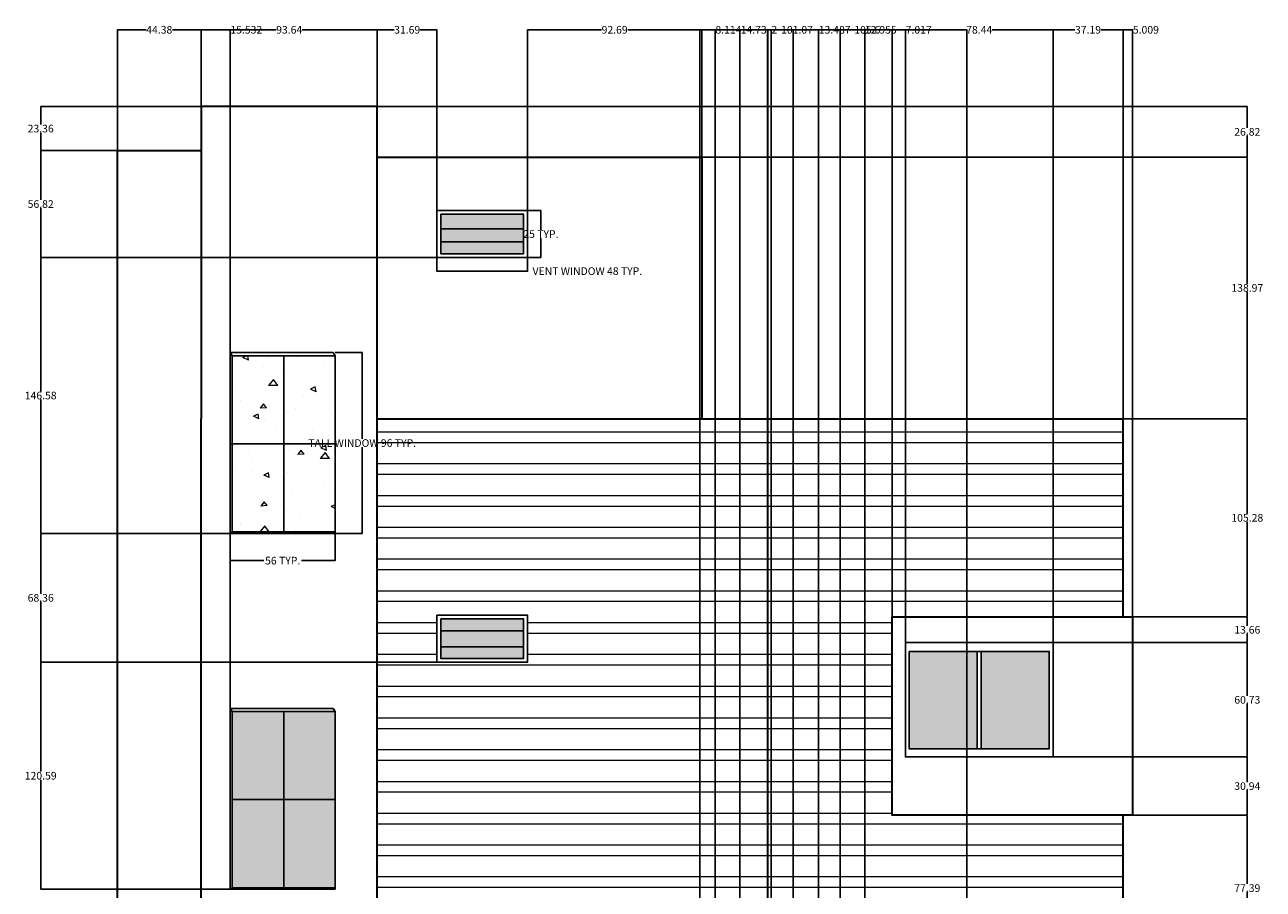
# Model space of a CAD drawing. Units: inches. Extents: x -35 to 623, y 74 to 964.
# Tile 3 of 3: x -35 to 623, y 505 to 964. Entities that reach past the tile are written whole.
import ezdxf

# ---------------------------------------------------------------- set-up
doc = ezdxf.new("R2010")
doc.units = ezdxf.units.IN
doc.header["$MEASUREMENT"] = 0
for name, color, linetype, lineweight in [('A-ANNO-DIMS', 2, 'Continuous', 18), ('A-ELEV', 7, 'Continuous', 35), ('A-ELEV-PATT', 8, 'Continuous', 13), ('A-GLAZ', 4, 'Continuous', 25)]:
    doc.layers.add(name, color=color, linetype=linetype, lineweight=lineweight)
doc.styles.get("Standard").update_dxf_attribs({"font": 'arial.ttf'})
doc.dimstyles.get("Standard").update_dxf_attribs({"dimtxt": 4.0625, "dimasz": 0.18, "dimexe": 0.18, "dimexo": 0.0625, "dimgap": 0.09, "dimtad": 0, "dimtih": 1, "dimtoh": 1, "dimdec": 4, "dimzin": 0, "dimdsep": 46, "dimlunit": 4, "dimtxsty": 'Standard', "dimcen": 0.09, "dimadec": 0, "dimazin": 0, "dimtfac": 1, "dimtdec": 4, "dimtofl": 0, "dimtmove": 0, "dimatfit": 3, "dimfxl": 1, "dimtolj": 1, "dimtzin": 0, "dimarcsym": 0})

# ---------------------------------------------------------------- blocks, each defined once
blk = doc.blocks.new('WIN-TALL-2X2')
for p, q in [((1.05, 94.39), (0, 96.09)), ((0, 96.09), (0, 0)), ((54.58, 96.06), (0, 96.06)), ((28.36, 94.39), (28.36, 0.82)), ((55.68, 94.39), (54.58, 96.06)), ((1.05, 0.82), (0, 0)), ((55.68, 0.82), (55.68, 0)), ((0, 0), (55.68, 0))]:
    blk.add_line(p, q)
blk.add_lwpolyline([(1.05, 94.39), (55.68, 94.39), (55.68, 0.82), (1.05, 0.82)], close=True)
blk = doc.blocks.new('VENT-FRAME')
for points in [[(0, 25.02), (48.03, 25.02), (48.03, 0), (0, 0)], [(2, 23.02), (46.03, 23.02), (46.03, 2), (2, 2)]]:
    blk.add_lwpolyline(points, close=True)
blk = doc.blocks.new('*D5')
at = {"layer": 'A-ANNO-DIMS', "color": 0, "lineweight": -2, "transparency": 16777216}
for p, q in [((129.92, 790.25), (144.45, 790.25)), ((144.27, 790.07), (144.27, 744.4)), ((144.27, 694.34), (144.27, 740.01)), ((129.92, 694.16), (144.45, 694.16))]:
    blk.add_line(p, q, dxfattribs=at)
at = {"layer": 'A-ANNO-DIMS', "color": 0, "transparency": 16777216}
for points in [[(144.24, 790.07), (144.3, 790.07), (144.27, 790.25)], [(144.24, 694.34), (144.3, 694.34), (144.27, 694.16)]]:
    blk.add_solid(points, dxfattribs=at)
at = {"layer": 'Defpoints', "color": 0, "transparency": 16777216}
for p in [(129.85, 790.25), (144.27, 790.25), (129.85, 694.16)]:
    blk.add_point(p, dxfattribs=at)
at = {"layer": 'A-ANNO-DIMS', "color": 0, "transparency": 16777216, "insert": (144.27, 742.2), "char_height": 4.0625, "attachment_point": 5}
blk.add_mtext('\\A1;TALL WINDOW 96 TYP.', dxfattribs=at)
blk = doc.blocks.new('*D6')
at = {"layer": 'A-ANNO-DIMS', "color": 0, "lineweight": -2, "transparency": 16777216}
for p, q in [((74.18, 694.1), (74.18, 679.56)), ((129.85, 694.1), (129.85, 679.56)), ((74.36, 679.74), (92.04, 679.74)), ((129.67, 679.74), (111.99, 679.74))]:
    blk.add_line(p, q, dxfattribs=at)
at = {"layer": 'A-ANNO-DIMS', "color": 0, "transparency": 16777216}
for points in [[(74.36, 679.77), (74.36, 679.71), (74.18, 679.74)], [(129.67, 679.77), (129.67, 679.71), (129.85, 679.74)]]:
    blk.add_solid(points, dxfattribs=at)
at = {"layer": 'Defpoints', "color": 0, "transparency": 16777216}
for p in [(74.18, 694.16), (129.85, 694.16), (129.85, 679.74)]:
    blk.add_point(p, dxfattribs=at)
at = {"layer": 'A-ANNO-DIMS', "color": 0, "transparency": 16777216, "insert": (102.02, 679.74), "char_height": 4.0625, "attachment_point": 5}
blk.add_mtext('\\A1;56 TYP.', dxfattribs=at)
blk = doc.blocks.new('*D7')
at = {"layer": 'A-ANNO-DIMS', "color": 0, "lineweight": -2, "transparency": 16777216}
for p, q in [((183.98, 840.67), (183.98, 833.35)), ((232.01, 840.67), (232.01, 833.35)), ((184.16, 833.53), (231.83, 833.53)), ((232.01, 833.53), (232.19, 833.53))]:
    blk.add_line(p, q, dxfattribs=at)
at = {"layer": 'A-ANNO-DIMS', "color": 0, "transparency": 16777216}
for points in [[(184.16, 833.56), (184.16, 833.5), (183.98, 833.53)], [(231.83, 833.56), (231.83, 833.5), (232.01, 833.53)]]:
    blk.add_solid(points, dxfattribs=at)
at = {"layer": 'Defpoints', "color": 0, "transparency": 16777216}
for p in [(183.98, 840.73), (232.01, 840.73), (232.01, 833.53)]:
    blk.add_point(p, dxfattribs=at)
at = {"layer": 'A-ANNO-DIMS', "color": 0, "transparency": 16777216, "insert": (263.87, 833.53), "char_height": 4.0625, "attachment_point": 5}
blk.add_mtext('\\A1;VENT WINDOW 48 TYP.', dxfattribs=at)
blk = doc.blocks.new('*D8')
at = {"layer": 'A-ANNO-DIMS', "color": 0, "lineweight": -2, "transparency": 16777216}
for p, q in [((232.07, 865.75), (239.39, 865.75)), ((239.21, 865.57), (239.21, 855.41)), ((239.21, 840.91), (239.21, 851.08)), ((232.07, 840.73), (239.39, 840.73))]:
    blk.add_line(p, q, dxfattribs=at)
at = {"layer": 'A-ANNO-DIMS', "color": 0, "transparency": 16777216}
for points in [[(239.18, 865.57), (239.24, 865.57), (239.21, 865.75)], [(239.18, 840.91), (239.24, 840.91), (239.21, 840.73)]]:
    blk.add_solid(points, dxfattribs=at)
at = {"layer": 'Defpoints', "color": 0, "transparency": 16777216}
for p in [(232.01, 865.75), (239.21, 865.75), (232.01, 840.73)]:
    blk.add_point(p, dxfattribs=at)
at = {"layer": 'A-ANNO-DIMS', "color": 0, "transparency": 16777216, "insert": (239.21, 853.24), "char_height": 4.0625, "attachment_point": 5}
blk.add_mtext('\\A1;25 TYP.', dxfattribs=at)
blk = doc.blocks.new('*D14')
at = {"layer": 'A-ANNO-DIMS', "color": 0, "lineweight": -2, "transparency": 16777216}
for p, q in [((14.26, 897.62), (14.26, 961.9)), ((14.44, 961.72), (29.42, 961.72)), ((58.47, 961.72), (43.48, 961.72)), ((58.65, 920.98), (58.65, 961.9))]:
    blk.add_line(p, q, dxfattribs=at)
at = {"layer": 'A-ANNO-DIMS', "color": 0, "transparency": 16777216}
for points in [[(14.44, 961.75), (14.44, 961.69), (14.26, 961.72)], [(58.47, 961.75), (58.47, 961.69), (58.65, 961.72)]]:
    blk.add_solid(points, dxfattribs=at)
at = {"layer": 'Defpoints', "color": 0, "transparency": 16777216}
for p in [(58.65, 961.72), (58.65, 920.92), (14.26, 897.56)]:
    blk.add_point(p, dxfattribs=at)
at = {"layer": 'A-ANNO-DIMS', "color": 0, "transparency": 16777216, "insert": (36.45, 961.72), "char_height": 4.062, "attachment_point": 5}
blk.add_mtext('\\A1;44.38', dxfattribs=at)
blk = doc.blocks.new('*D15')
at = {"layer": 'A-ANNO-DIMS', "color": 0, "lineweight": -2, "transparency": 16777216}
for p, q in [((58.65, 920.98), (58.65, 961.9)), ((58.83, 961.72), (98.53, 961.72)), ((152.11, 961.72), (112.4, 961.72)), ((152.29, 920.98), (152.29, 961.9))]:
    blk.add_line(p, q, dxfattribs=at)
at = {"layer": 'A-ANNO-DIMS', "color": 0, "transparency": 16777216}
for points in [[(58.83, 961.75), (58.83, 961.69), (58.65, 961.72)], [(152.11, 961.75), (152.11, 961.69), (152.29, 961.72)]]:
    blk.add_solid(points, dxfattribs=at)
at = {"layer": 'Defpoints', "color": 0, "transparency": 16777216}
for p in [(152.29, 961.72), (58.65, 920.92), (152.29, 920.92)]:
    blk.add_point(p, dxfattribs=at)
at = {"layer": 'A-ANNO-DIMS', "color": 0, "transparency": 16777216, "insert": (105.47, 961.72), "char_height": 4.062, "attachment_point": 5}
blk.add_mtext('\\A1;93.64', dxfattribs=at)
blk = doc.blocks.new('*D16')
at = {"layer": 'A-ANNO-DIMS', "color": 0, "lineweight": -2, "transparency": 16777216}
for p, q in [((152.29, 894.16), (152.29, 961.9)), ((152.47, 961.72), (161.19, 961.72)), ((183.8, 961.72), (175.08, 961.72)), ((183.98, 865.81), (183.98, 961.9))]:
    blk.add_line(p, q, dxfattribs=at)
at = {"layer": 'A-ANNO-DIMS', "color": 0, "transparency": 16777216}
for points in [[(152.47, 961.75), (152.47, 961.69), (152.29, 961.72)], [(183.8, 961.75), (183.8, 961.69), (183.98, 961.72)]]:
    blk.add_solid(points, dxfattribs=at)
at = {"layer": 'Defpoints', "color": 0, "transparency": 16777216}
for p in [(183.98, 961.72), (152.29, 894.1), (183.98, 865.75)]:
    blk.add_point(p, dxfattribs=at)
at = {"layer": 'A-ANNO-DIMS', "color": 0, "transparency": 16777216, "insert": (168.14, 961.72), "char_height": 4.062, "attachment_point": 5}
blk.add_mtext('\\A1;31.69', dxfattribs=at)
blk = doc.blocks.new('*D17')
at = {"layer": 'A-ANNO-DIMS', "color": 0, "lineweight": -2, "transparency": 16777216}
for p, q in [((232.01, 865.81), (232.01, 961.9)), ((232.19, 961.72), (271.4, 961.72)), ((324.52, 961.72), (285.3, 961.72)), ((324.7, 894.16), (324.7, 961.9))]:
    blk.add_line(p, q, dxfattribs=at)
at = {"layer": 'A-ANNO-DIMS', "color": 0, "transparency": 16777216}
for points in [[(232.19, 961.75), (232.19, 961.69), (232.01, 961.72)], [(324.52, 961.75), (324.52, 961.69), (324.7, 961.72)]]:
    blk.add_solid(points, dxfattribs=at)
at = {"layer": 'Defpoints', "color": 0, "transparency": 16777216}
for p in [(324.7, 961.72), (324.7, 894.1), (232.01, 865.75)]:
    blk.add_point(p, dxfattribs=at)
at = {"layer": 'A-ANNO-DIMS', "color": 0, "transparency": 16777216, "insert": (278.35, 961.72), "char_height": 4.062, "attachment_point": 5}
blk.add_mtext('\\A1;92.69', dxfattribs=at)
blk = doc.blocks.new('*D18')
at = {"layer": 'A-ANNO-DIMS', "color": 0, "lineweight": -2, "transparency": 16777216}
for p, q in [((324.7, 755.19), (324.7, 961.9)), ((324.88, 961.72), (366.9, 961.72)), ((425.59, 961.72), (383.56, 961.72)), ((425.77, 649.91), (425.77, 961.9))]:
    blk.add_line(p, q, dxfattribs=at)
at = {"layer": 'A-ANNO-DIMS', "color": 0, "transparency": 16777216}
for points in [[(324.88, 961.75), (324.88, 961.69), (324.7, 961.72)], [(425.59, 961.75), (425.59, 961.69), (425.77, 961.72)]]:
    blk.add_solid(points, dxfattribs=at)
at = {"layer": 'Defpoints', "color": 0, "transparency": 16777216}
for p in [(425.77, 961.72), (324.7, 755.13), (425.77, 649.84)]:
    blk.add_point(p, dxfattribs=at)
at = {"layer": 'A-ANNO-DIMS', "color": 0, "transparency": 16777216, "insert": (375.23, 961.72), "char_height": 4.062, "attachment_point": 5}
blk.add_mtext('\\A1;101.07', dxfattribs=at)
blk = doc.blocks.new('*D19')
at = {"layer": 'A-ANNO-DIMS', "color": 0, "lineweight": -2, "transparency": 16777216}
for p, q in [((425.77, 649.91), (425.77, 961.9)), ((425.95, 961.72), (432.61, 961.72)), ((432.79, 636.25), (432.79, 961.9)), ((432.79, 961.72), (432.97, 961.72))]:
    blk.add_line(p, q, dxfattribs=at)
at = {"layer": 'A-ANNO-DIMS', "color": 0, "transparency": 16777216}
for points in [[(425.95, 961.75), (425.95, 961.69), (425.77, 961.72)], [(432.61, 961.75), (432.61, 961.69), (432.79, 961.72)]]:
    blk.add_solid(points, dxfattribs=at)
at = {"layer": 'Defpoints', "color": 0, "transparency": 16777216}
for p in [(432.79, 961.72), (425.77, 649.84), (432.79, 636.18)]:
    blk.add_point(p, dxfattribs=at)
at = {"layer": 'A-ANNO-DIMS', "color": 0, "transparency": 16777216, "insert": (439.89, 961.72), "char_height": 4.062, "attachment_point": 5}
blk.add_mtext('\\A1;7.017', dxfattribs=at)
blk = doc.blocks.new('*D20')
at = {"layer": 'A-ANNO-DIMS', "color": 0, "lineweight": -2, "transparency": 16777216}
for p, q in [((432.79, 636.25), (432.79, 961.9)), ((432.97, 961.72), (465.09, 961.72)), ((511.05, 961.72), (478.93, 961.72)), ((511.23, 636.25), (511.23, 961.9))]:
    blk.add_line(p, q, dxfattribs=at)
at = {"layer": 'A-ANNO-DIMS', "color": 0, "transparency": 16777216}
for points in [[(432.97, 961.75), (432.97, 961.69), (432.79, 961.72)], [(511.05, 961.75), (511.05, 961.69), (511.23, 961.72)]]:
    blk.add_solid(points, dxfattribs=at)
at = {"layer": 'Defpoints', "color": 0, "transparency": 16777216}
for p in [(511.23, 961.72), (432.79, 636.18), (511.23, 636.18)]:
    blk.add_point(p, dxfattribs=at)
at = {"layer": 'A-ANNO-DIMS', "color": 0, "transparency": 16777216, "insert": (472.01, 961.72), "char_height": 4.062, "attachment_point": 5}
blk.add_mtext('\\A1;78.44', dxfattribs=at)
blk = doc.blocks.new('*D21')
at = {"layer": 'A-ANNO-DIMS', "color": 0, "lineweight": -2, "transparency": 16777216}
for p, q in [((511.23, 636.25), (511.23, 961.9)), ((511.41, 961.72), (522.87, 961.72)), ((548.24, 961.72), (536.77, 961.72)), ((548.42, 755.19), (548.42, 961.9))]:
    blk.add_line(p, q, dxfattribs=at)
at = {"layer": 'A-ANNO-DIMS', "color": 0, "transparency": 16777216}
for points in [[(511.41, 961.75), (511.41, 961.69), (511.23, 961.72)], [(548.24, 961.75), (548.24, 961.69), (548.42, 961.72)]]:
    blk.add_solid(points, dxfattribs=at)
at = {"layer": 'Defpoints', "color": 0, "transparency": 16777216}
for p in [(548.42, 961.72), (548.42, 755.13), (511.23, 636.18)]:
    blk.add_point(p, dxfattribs=at)
at = {"layer": 'A-ANNO-DIMS', "color": 0, "transparency": 16777216, "insert": (529.82, 961.72), "char_height": 4.062, "attachment_point": 5}
blk.add_mtext('\\A1;37.19', dxfattribs=at)
blk = doc.blocks.new('*D22')
at = {"layer": 'A-ANNO-DIMS', "color": 0, "lineweight": -2, "transparency": 16777216}
for p, q in [((548.42, 755.19), (548.42, 961.9)), ((548.6, 961.72), (553.25, 961.72)), ((553.43, 649.91), (553.43, 961.9)), ((553.43, 961.72), (553.61, 961.72))]:
    blk.add_line(p, q, dxfattribs=at)
at = {"layer": 'A-ANNO-DIMS', "color": 0, "transparency": 16777216}
for points in [[(548.6, 961.75), (548.6, 961.69), (548.42, 961.72)], [(553.25, 961.75), (553.25, 961.69), (553.43, 961.72)]]:
    blk.add_solid(points, dxfattribs=at)
at = {"layer": 'Defpoints', "color": 0, "transparency": 16777216}
for p in [(553.43, 961.72), (548.42, 755.13), (553.43, 649.84)]:
    blk.add_point(p, dxfattribs=at)
at = {"layer": 'A-ANNO-DIMS', "color": 0, "transparency": 16777216, "insert": (560.56, 961.72), "char_height": 4.062, "attachment_point": 5}
blk.add_mtext('\\A1;5.009', dxfattribs=at)
blk = doc.blocks.new('*D26')
at = {"layer": 'A-ANNO-DIMS', "color": 0, "lineweight": -2, "transparency": 16777216}
for p, q in [((553.49, 544.52), (614.62, 544.52)), ((614.44, 544.34), (614.44, 507.99)), ((614.44, 467.31), (614.44, 503.66)), ((548.48, 467.13), (614.62, 467.13))]:
    blk.add_line(p, q, dxfattribs=at)
at = {"layer": 'A-ANNO-DIMS', "color": 0, "transparency": 16777216}
for points in [[(614.41, 544.34), (614.47, 544.34), (614.44, 544.52)], [(614.41, 467.31), (614.47, 467.31), (614.44, 467.13)]]:
    blk.add_solid(points, dxfattribs=at)
at = {"layer": 'Defpoints', "color": 0, "transparency": 16777216}
for p in [(553.43, 544.52), (614.44, 544.52), (548.42, 467.13)]:
    blk.add_point(p, dxfattribs=at)
at = {"layer": 'A-ANNO-DIMS', "color": 0, "transparency": 16777216, "insert": (614.44, 505.82), "char_height": 4.062, "attachment_point": 5}
blk.add_mtext('\\A1;77.39', dxfattribs=at)
blk = doc.blocks.new('*D27')
at = {"layer": 'A-ANNO-DIMS', "color": 0, "lineweight": -2, "transparency": 16777216}
for p, q in [((511.29, 575.46), (614.62, 575.46)), ((614.44, 575.28), (614.44, 562.15)), ((614.44, 544.7), (614.44, 557.82)), ((553.49, 544.52), (614.62, 544.52))]:
    blk.add_line(p, q, dxfattribs=at)
at = {"layer": 'A-ANNO-DIMS', "color": 0, "transparency": 16777216}
for points in [[(614.41, 575.28), (614.47, 575.28), (614.44, 575.46)], [(614.41, 544.7), (614.47, 544.7), (614.44, 544.52)]]:
    blk.add_solid(points, dxfattribs=at)
at = {"layer": 'Defpoints', "color": 0, "transparency": 16777216}
for p in [(511.23, 575.46), (614.44, 575.46), (553.43, 544.52)]:
    blk.add_point(p, dxfattribs=at)
at = {"layer": 'A-ANNO-DIMS', "color": 0, "transparency": 16777216, "insert": (614.44, 559.99), "char_height": 4.062, "attachment_point": 5}
blk.add_mtext('\\A1;30.94', dxfattribs=at)
blk = doc.blocks.new('*D28')
at = {"layer": 'A-ANNO-DIMS', "color": 0, "lineweight": -2, "transparency": 16777216}
for p, q in [((511.29, 636.18), (614.62, 636.18)), ((614.44, 636), (614.44, 607.98)), ((614.44, 575.64), (614.44, 603.65)), ((511.29, 575.46), (614.62, 575.46))]:
    blk.add_line(p, q, dxfattribs=at)
at = {"layer": 'A-ANNO-DIMS', "color": 0, "transparency": 16777216}
for points in [[(614.41, 636), (614.47, 636), (614.44, 636.18)], [(614.41, 575.64), (614.47, 575.64), (614.44, 575.46)]]:
    blk.add_solid(points, dxfattribs=at)
at = {"layer": 'Defpoints', "color": 0, "transparency": 16777216}
for p in [(511.23, 636.18), (614.44, 636.18), (511.23, 575.46)]:
    blk.add_point(p, dxfattribs=at)
at = {"layer": 'A-ANNO-DIMS', "color": 0, "transparency": 16777216, "insert": (614.44, 605.82), "char_height": 4.062, "attachment_point": 5}
blk.add_mtext('\\A1;60.73', dxfattribs=at)
blk = doc.blocks.new('*D29')
at = {"layer": 'A-ANNO-DIMS', "color": 0, "lineweight": -2, "transparency": 16777216}
for p, q in [((553.49, 649.84), (614.62, 649.84)), ((614.44, 649.66), (614.44, 645.18)), ((614.44, 636.36), (614.44, 640.85)), ((511.29, 636.18), (614.62, 636.18))]:
    blk.add_line(p, q, dxfattribs=at)
at = {"layer": 'A-ANNO-DIMS', "color": 0, "transparency": 16777216}
for points in [[(614.41, 649.66), (614.47, 649.66), (614.44, 649.84)], [(614.41, 636.36), (614.47, 636.36), (614.44, 636.18)]]:
    blk.add_solid(points, dxfattribs=at)
at = {"layer": 'Defpoints', "color": 0, "transparency": 16777216}
for p in [(553.43, 649.84), (614.44, 649.84), (511.23, 636.18)]:
    blk.add_point(p, dxfattribs=at)
at = {"layer": 'A-ANNO-DIMS', "color": 0, "transparency": 16777216, "insert": (614.44, 643.01), "char_height": 4.062, "attachment_point": 5}
blk.add_mtext('\\A1;13.66', dxfattribs=at)
blk = doc.blocks.new('*D30')
at = {"layer": 'A-ANNO-DIMS', "color": 0, "lineweight": -2, "transparency": 16777216}
for p, q in [((548.48, 755.13), (614.62, 755.13)), ((614.44, 754.95), (614.44, 704.65)), ((614.44, 650.02), (614.44, 700.32)), ((553.49, 649.84), (614.62, 649.84))]:
    blk.add_line(p, q, dxfattribs=at)
at = {"layer": 'A-ANNO-DIMS', "color": 0, "transparency": 16777216}
for points in [[(614.41, 754.95), (614.47, 754.95), (614.44, 755.13)], [(614.41, 650.02), (614.47, 650.02), (614.44, 649.84)]]:
    blk.add_solid(points, dxfattribs=at)
at = {"layer": 'Defpoints', "color": 0, "transparency": 16777216}
for p in [(548.42, 755.13), (614.44, 755.13), (553.43, 649.84)]:
    blk.add_point(p, dxfattribs=at)
at = {"layer": 'A-ANNO-DIMS', "color": 0, "transparency": 16777216, "insert": (614.44, 702.49), "char_height": 4.062, "attachment_point": 5}
blk.add_mtext('\\A1;105.28', dxfattribs=at)
blk = doc.blocks.new('*D31')
at = {"layer": 'A-ANNO-DIMS', "color": 0, "lineweight": -2, "transparency": 16777216}
for p, q in [((324.76, 894.1), (614.62, 894.1)), ((614.44, 893.92), (614.44, 826.78)), ((614.44, 755.31), (614.44, 822.45)), ((548.48, 755.13), (614.62, 755.13))]:
    blk.add_line(p, q, dxfattribs=at)
at = {"layer": 'A-ANNO-DIMS', "color": 0, "transparency": 16777216}
for points in [[(614.41, 893.92), (614.47, 893.92), (614.44, 894.1)], [(614.41, 755.31), (614.47, 755.31), (614.44, 755.13)]]:
    blk.add_solid(points, dxfattribs=at)
at = {"layer": 'Defpoints', "color": 0, "transparency": 16777216}
for p in [(324.7, 894.1), (614.44, 894.1), (548.42, 755.13)]:
    blk.add_point(p, dxfattribs=at)
at = {"layer": 'A-ANNO-DIMS', "color": 0, "transparency": 16777216, "insert": (614.44, 824.61), "char_height": 4.062, "attachment_point": 5}
blk.add_mtext('\\A1;138.97', dxfattribs=at)
blk = doc.blocks.new('*D32')
at = {"layer": 'A-ANNO-DIMS', "color": 0, "lineweight": -2, "transparency": 16777216}
for p, q in [((152.35, 920.92), (614.62, 920.92)), ((614.44, 920.74), (614.44, 909.67)), ((614.44, 894.28), (614.44, 905.34)), ((324.76, 894.1), (614.62, 894.1))]:
    blk.add_line(p, q, dxfattribs=at)
at = {"layer": 'A-ANNO-DIMS', "color": 0, "transparency": 16777216}
for points in [[(614.41, 920.74), (614.47, 920.74), (614.44, 920.92)], [(614.41, 894.28), (614.47, 894.28), (614.44, 894.1)]]:
    blk.add_solid(points, dxfattribs=at)
at = {"layer": 'Defpoints', "color": 0, "transparency": 16777216}
for p in [(152.29, 920.92), (614.44, 920.92), (324.7, 894.1)]:
    blk.add_point(p, dxfattribs=at)
at = {"layer": 'A-ANNO-DIMS', "color": 0, "transparency": 16777216, "insert": (614.44, 907.51), "char_height": 4.062, "attachment_point": 5}
blk.add_mtext('\\A1;26.82', dxfattribs=at)
blk = doc.blocks.new('*D36')
at = {"layer": 'A-ANNO-DIMS', "color": 0, "lineweight": -2, "transparency": 16777216}
for p, q in [((183.92, 625.8), (-26.72, 625.8)), ((-26.54, 625.62), (-26.54, 567.67)), ((-26.54, 505.39), (-26.54, 563.34)), ((74.11, 505.21), (-26.72, 505.21))]:
    blk.add_line(p, q, dxfattribs=at)
at = {"layer": 'A-ANNO-DIMS', "color": 0, "transparency": 16777216}
for points in [[(-26.57, 625.62), (-26.51, 625.62), (-26.54, 625.8)], [(-26.57, 505.39), (-26.51, 505.39), (-26.54, 505.21)]]:
    blk.add_solid(points, dxfattribs=at)
at = {"layer": 'Defpoints', "color": 0, "transparency": 16777216}
for p in [(-26.54, 625.8), (183.98, 625.8), (74.18, 505.21)]:
    blk.add_point(p, dxfattribs=at)
at = {"layer": 'A-ANNO-DIMS', "color": 0, "transparency": 16777216, "insert": (-26.54, 565.5), "char_height": 4.062, "attachment_point": 5}
blk.add_mtext('\\A1;120.59', dxfattribs=at)
blk = doc.blocks.new('*D37')
at = {"layer": 'A-ANNO-DIMS', "color": 0, "lineweight": -2, "transparency": 16777216}
for p, q in [((74.11, 694.16), (-26.72, 694.16)), ((-26.54, 693.98), (-26.54, 662.14)), ((-26.54, 625.98), (-26.54, 657.81)), ((183.92, 625.8), (-26.72, 625.8))]:
    blk.add_line(p, q, dxfattribs=at)
at = {"layer": 'A-ANNO-DIMS', "color": 0, "transparency": 16777216}
for points in [[(-26.57, 693.98), (-26.51, 693.98), (-26.54, 694.16)], [(-26.57, 625.98), (-26.51, 625.98), (-26.54, 625.8)]]:
    blk.add_solid(points, dxfattribs=at)
at = {"layer": 'Defpoints', "color": 0, "transparency": 16777216}
for p in [(-26.54, 694.16), (74.18, 694.16), (183.98, 625.8)]:
    blk.add_point(p, dxfattribs=at)
at = {"layer": 'A-ANNO-DIMS', "color": 0, "transparency": 16777216, "insert": (-26.54, 659.98), "char_height": 4.062, "attachment_point": 5}
blk.add_mtext('\\A1;68.36', dxfattribs=at)
blk = doc.blocks.new('*D38')
at = {"layer": 'A-ANNO-DIMS', "color": 0, "lineweight": -2, "transparency": 16777216}
for p, q in [((183.92, 840.73), (-26.72, 840.73)), ((-26.54, 840.55), (-26.54, 769.61)), ((-26.54, 694.34), (-26.54, 765.28)), ((74.11, 694.16), (-26.72, 694.16))]:
    blk.add_line(p, q, dxfattribs=at)
at = {"layer": 'A-ANNO-DIMS', "color": 0, "transparency": 16777216}
for points in [[(-26.57, 840.55), (-26.51, 840.55), (-26.54, 840.73)], [(-26.57, 694.34), (-26.51, 694.34), (-26.54, 694.16)]]:
    blk.add_solid(points, dxfattribs=at)
at = {"layer": 'Defpoints', "color": 0, "transparency": 16777216}
for p in [(-26.54, 840.73), (183.98, 840.73), (74.18, 694.16)]:
    blk.add_point(p, dxfattribs=at)
at = {"layer": 'A-ANNO-DIMS', "color": 0, "transparency": 16777216, "insert": (-26.54, 767.45), "char_height": 4.062, "attachment_point": 5}
blk.add_mtext('\\A1;146.58', dxfattribs=at)
blk = doc.blocks.new('*D39')
at = {"layer": 'A-ANNO-DIMS', "color": 0, "lineweight": -2, "transparency": 16777216}
for p, q in [((14.2, 897.56), (-26.72, 897.56)), ((-26.54, 897.38), (-26.54, 871.31)), ((-26.54, 840.91), (-26.54, 866.98)), ((183.92, 840.73), (-26.72, 840.73))]:
    blk.add_line(p, q, dxfattribs=at)
at = {"layer": 'A-ANNO-DIMS', "color": 0, "transparency": 16777216}
for points in [[(-26.57, 897.38), (-26.51, 897.38), (-26.54, 897.56)], [(-26.57, 840.91), (-26.51, 840.91), (-26.54, 840.73)]]:
    blk.add_solid(points, dxfattribs=at)
at = {"layer": 'Defpoints', "color": 0, "transparency": 16777216}
for p in [(-26.54, 897.56), (14.26, 897.56), (183.98, 840.73)]:
    blk.add_point(p, dxfattribs=at)
at = {"layer": 'A-ANNO-DIMS', "color": 0, "transparency": 16777216, "insert": (-26.54, 869.15), "char_height": 4.062, "attachment_point": 5}
blk.add_mtext('\\A1;56.82', dxfattribs=at)
blk = doc.blocks.new('*D40')
at = {"layer": 'A-ANNO-DIMS', "color": 0, "lineweight": -2, "transparency": 16777216}
for p, q in [((58.58, 920.92), (-26.72, 920.92)), ((-26.54, 920.74), (-26.54, 911.4)), ((-26.54, 897.74), (-26.54, 907.07)), ((14.2, 897.56), (-26.72, 897.56))]:
    blk.add_line(p, q, dxfattribs=at)
at = {"layer": 'A-ANNO-DIMS', "color": 0, "transparency": 16777216}
for points in [[(-26.57, 920.74), (-26.51, 920.74), (-26.54, 920.92)], [(-26.57, 897.74), (-26.51, 897.74), (-26.54, 897.56)]]:
    blk.add_solid(points, dxfattribs=at)
at = {"layer": 'Defpoints', "color": 0, "transparency": 16777216}
for p in [(-26.54, 920.92), (58.65, 920.92), (14.26, 897.56)]:
    blk.add_point(p, dxfattribs=at)
at = {"layer": 'A-ANNO-DIMS', "color": 0, "transparency": 16777216, "insert": (-26.54, 909.24), "char_height": 4.062, "attachment_point": 5}
blk.add_mtext('\\A1;23.36', dxfattribs=at)
blk = doc.blocks.new('*D41')
at = {"layer": 'A-ANNO-DIMS', "color": 0, "lineweight": -2, "transparency": 16777216}
for p, q in [((58.65, 611.19), (58.65, 961.9)), ((58.83, 961.72), (74, 961.72)), ((74.18, 601.33), (74.18, 961.9)), ((74.18, 961.72), (74.36, 961.72))]:
    blk.add_line(p, q, dxfattribs=at)
at = {"layer": 'A-ANNO-DIMS', "color": 0, "transparency": 16777216}
for points in [[(58.83, 961.75), (58.83, 961.69), (58.65, 961.72)], [(74, 961.75), (74, 961.69), (74.18, 961.72)]]:
    blk.add_solid(points, dxfattribs=at)
at = {"layer": 'Defpoints', "color": 0, "transparency": 16777216}
for p in [(74.18, 961.72), (58.65, 611.13), (74.18, 601.27)]:
    blk.add_point(p, dxfattribs=at)
at = {"layer": 'A-ANNO-DIMS', "color": 0, "transparency": 16777216, "insert": (82.67, 961.72), "char_height": 4.062, "attachment_point": 5}
blk.add_mtext('\\A1;15.532', dxfattribs=at)
blk = doc.blocks.new('*D58')
at = {"layer": 'A-ANNO-DIMS', "color": 0, "lineweight": -2, "transparency": 16777216}
for p, q in [((323.56, 323.19), (323.56, 961.9)), ((323.74, 961.72), (331.5, 961.72)), ((331.68, 323.19), (331.68, 961.9)), ((331.68, 961.72), (331.86, 961.72))]:
    blk.add_line(p, q, dxfattribs=at)
at = {"layer": 'A-ANNO-DIMS', "color": 0, "transparency": 16777216}
for points in [[(323.74, 961.75), (323.74, 961.69), (323.56, 961.72)], [(331.5, 961.75), (331.5, 961.69), (331.68, 961.72)]]:
    blk.add_solid(points, dxfattribs=at)
at = {"layer": 'Defpoints', "color": 0, "transparency": 16777216}
for p in [(331.68, 961.72), (323.56, 323.13), (331.68, 323.13)]:
    blk.add_point(p, dxfattribs=at)
at = {"layer": 'A-ANNO-DIMS', "color": 0, "transparency": 16777216, "insert": (338.8, 961.72), "char_height": 4.062, "attachment_point": 5}
blk.add_mtext('\\A1;8.114', dxfattribs=at)
blk = doc.blocks.new('*D59')
at = {"layer": 'A-ANNO-DIMS', "color": 0, "lineweight": -2, "transparency": 16777216}
for p, q in [((344.83, 323.19), (344.83, 961.9)), ((345.01, 961.72), (345.44, 961.72)), ((359.38, 961.72), (358.95, 961.72)), ((359.56, 323.19), (359.56, 961.9))]:
    blk.add_line(p, q, dxfattribs=at)
at = {"layer": 'A-ANNO-DIMS', "color": 0, "transparency": 16777216}
for points in [[(345.01, 961.75), (345.01, 961.69), (344.83, 961.72)], [(359.38, 961.75), (359.38, 961.69), (359.56, 961.72)]]:
    blk.add_solid(points, dxfattribs=at)
at = {"layer": 'Defpoints', "color": 0, "transparency": 16777216}
for p in [(359.56, 961.72), (344.83, 323.13), (359.56, 323.13)]:
    blk.add_point(p, dxfattribs=at)
at = {"layer": 'A-ANNO-DIMS', "color": 0, "transparency": 16777216, "insert": (352.19, 961.72), "char_height": 4.062, "attachment_point": 5}
blk.add_mtext('\\A1;14.73', dxfattribs=at)
blk = doc.blocks.new('*D60')
at = {"layer": 'A-ANNO-DIMS', "color": 0, "lineweight": -2, "transparency": 16777216}
for p, q in [((359.56, 323.19), (359.56, 961.9)), ((359.74, 961.72), (361.38, 961.72)), ((361.56, 323.19), (361.56, 961.9)), ((361.56, 961.72), (361.74, 961.72))]:
    blk.add_line(p, q, dxfattribs=at)
at = {"layer": 'A-ANNO-DIMS', "color": 0, "transparency": 16777216}
for points in [[(359.74, 961.75), (359.74, 961.69), (359.56, 961.72)], [(361.38, 961.75), (361.38, 961.69), (361.56, 961.72)]]:
    blk.add_solid(points, dxfattribs=at)
at = {"layer": 'Defpoints', "color": 0, "transparency": 16777216}
for p in [(361.56, 961.72), (359.56, 323.13), (361.56, 323.13)]:
    blk.add_point(p, dxfattribs=at)
at = {"layer": 'A-ANNO-DIMS', "color": 0, "transparency": 16777216, "insert": (363.17, 961.72), "char_height": 4.062, "attachment_point": 5}
blk.add_mtext('\\A1;2', dxfattribs=at)
blk = doc.blocks.new('*D61')
at = {"layer": 'A-ANNO-DIMS', "color": 0, "lineweight": -2, "transparency": 16777216}
for p, q in [((373.22, 323.19), (373.22, 961.9)), ((373.4, 961.72), (386.53, 961.72)), ((386.71, 323.19), (386.71, 961.9)), ((386.71, 961.72), (386.89, 961.72))]:
    blk.add_line(p, q, dxfattribs=at)
at = {"layer": 'A-ANNO-DIMS', "color": 0, "transparency": 16777216}
for points in [[(373.4, 961.75), (373.4, 961.69), (373.22, 961.72)], [(386.53, 961.75), (386.53, 961.69), (386.71, 961.72)]]:
    blk.add_solid(points, dxfattribs=at)
at = {"layer": 'Defpoints', "color": 0, "transparency": 16777216}
for p in [(386.71, 961.72), (373.22, 323.13), (386.71, 323.13)]:
    blk.add_point(p, dxfattribs=at)
at = {"layer": 'A-ANNO-DIMS', "color": 0, "transparency": 16777216, "insert": (395.22, 961.72), "char_height": 4.062, "attachment_point": 5}
blk.add_mtext('\\A1;13.487', dxfattribs=at)
blk = doc.blocks.new('*D62')
at = {"layer": 'A-ANNO-DIMS', "color": 0, "lineweight": -2, "transparency": 16777216}
for p, q in [((398.24, 323.19), (398.24, 961.9)), ((398.42, 961.72), (411.02, 961.72)), ((411.2, 323.19), (411.2, 961.9)), ((411.2, 961.72), (411.38, 961.72))]:
    blk.add_line(p, q, dxfattribs=at)
at = {"layer": 'A-ANNO-DIMS', "color": 0, "transparency": 16777216}
for points in [[(398.42, 961.75), (398.42, 961.69), (398.24, 961.72)], [(411.02, 961.75), (411.02, 961.69), (411.2, 961.72)]]:
    blk.add_solid(points, dxfattribs=at)
at = {"layer": 'Defpoints', "color": 0, "transparency": 16777216}
for p in [(411.2, 961.72), (398.24, 323.13), (411.2, 323.13)]:
    blk.add_point(p, dxfattribs=at)
at = {"layer": 'A-ANNO-DIMS', "color": 0, "transparency": 16777216, "insert": (419.73, 961.72), "char_height": 4.062, "attachment_point": 5}
blk.add_mtext('\\A1;12.955', dxfattribs=at)
blk = doc.blocks.new('*D70')
at = {"layer": 'A-ANNO-DIMS', "color": 0, "lineweight": -2, "transparency": 16777216}
for p, q in [((359.79, 445.41), (359.79, 961.9)), ((359.97, 961.72), (405.84, 961.72)), ((465.22, 961.72), (419.34, 961.72)), ((465.4, 445.41), (465.4, 961.9))]:
    blk.add_line(p, q, dxfattribs=at)
at = {"layer": 'A-ANNO-DIMS', "color": 0, "transparency": 16777216}
for points in [[(359.97, 961.75), (359.97, 961.69), (359.79, 961.72)], [(465.22, 961.75), (465.22, 961.69), (465.4, 961.72)]]:
    blk.add_solid(points, dxfattribs=at)
at = {"layer": 'Defpoints', "color": 0, "transparency": 16777216}
for p in [(465.4, 961.72), (359.79, 445.34), (465.4, 445.34)]:
    blk.add_point(p, dxfattribs=at)
at = {"layer": 'A-ANNO-DIMS', "color": 0, "transparency": 16777216, "insert": (412.59, 961.72), "char_height": 4.062, "attachment_point": 5}
blk.add_mtext('\\A1;105.6', dxfattribs=at)

msp = doc.modelspace()

# ---------------------------------------------------------------- hatches: boundary and pattern name
at = {"layer": 'A-ELEV-PATT'}
h = msp.add_hatch(color=256, dxfattribs=at)
h.dxf.hatch_style = 1
h.set_gradient(color2=(99, 100, 102))
h.paths.add_polyline_path([(471.0064, 631.4927), (434.7868, 631.4927), (434.7868, 579.8536), (471.0064, 579.8536)])
h.paths.add_polyline_path([(509.226, 631.4927), (473.0064, 631.4927), (473.0064, 579.8536), (509.226, 579.8536)])
h.paths.add_polyline_path([(449.3739, 427.1438), (413.1543, 427.1438), (413.1543, 380.7902), (449.3739, 380.7902)])
h.paths.add_polyline_path([(411.1543, 427.1438), (374.9347, 427.1438), (374.9347, 380.7902), (411.1543, 380.7902)])
h.paths.add_polyline_path([(374.9294, 263.937), (338.7098, 263.937), (338.7098, 217.5834), (374.9294, 217.5834)])
h.paths.add_polyline_path([(413.1491, 263.937), (376.9294, 263.937), (376.9294, 217.5834), (413.1491, 217.5834)])
h.paths.add_polyline_path([(230.0086, 434.3669), (185.9817, 434.3669), (185.9817, 426.9441), (230.0086, 426.9441)])
h.paths.add_polyline_path([(230.0086, 443.5602), (185.9817, 443.5602), (185.9817, 434.3669), (230.0086, 434.3669)])
h.paths.add_polyline_path([(230.0086, 426.9441), (185.9817, 426.9441), (185.9817, 422.542), (230.0086, 422.542)])
h.paths.add_polyline_path([(230.0086, 648.8148), (185.9817, 648.8148), (185.9817, 642.5298), (230.0086, 642.5298)])
h.paths.add_polyline_path([(230.0086, 642.5298), (185.9817, 642.5298), (185.9817, 633.9381), (230.0086, 633.9381)])
h.paths.add_polyline_path([(230.0086, 633.9381), (185.9817, 633.9381), (185.9817, 627.7966), (230.0086, 627.7966)])
h.paths.add_polyline_path([(230.0086, 863.7512), (185.9817, 863.7512), (185.9817, 856.0022), (230.0086, 856.0022)])
h.paths.add_polyline_path([(230.0086, 856.0022), (185.9817, 856.0022), (185.9817, 849.1652), (230.0086, 849.1652)])
h.paths.add_polyline_path([(230.0086, 849.1652), (185.9817, 849.1652), (185.9817, 842.733), (230.0086, 842.733)])
h = msp.add_hatch(dxfattribs=at)
h.set_pattern_fill('AR-CONC', color=256, scale=4.4, angle=134)
h.paths.add_polyline_path([(129.855, 788.5505), (102.5419, 788.5505), (102.5419, 741.7655), (129.855, 741.7655)])
h.paths.add_polyline_path([(102.5419, 788.5505), (75.2288, 788.5505), (75.2288, 741.7655), (102.5419, 741.7655)])
h.paths.add_polyline_path([(129.855, 741.7655), (102.5419, 741.7655), (102.5419, 694.9806), (129.855, 694.9806)])
h.paths.add_polyline_path([(102.5419, 741.7655), (75.2288, 741.7655), (75.2288, 694.9806), (102.5419, 694.9806)])
h = msp.add_hatch(dxfattribs=at)
h.set_pattern_fill('ANSI32', color=256, scale=45, angle=135)
h.paths.add_polyline_path([(548.4175, 755.1261), (152.2908, 755.1261), (152.2908, 611.1261), (152.2908, 467.1261), (548.4175, 467.1261), (548.4175, 544.5164), (425.7698, 544.5164), (425.7698, 649.844), (548.4175, 649.844)])
h.paths.add_polyline_path([(232.0086, 650.8148), (232.0086, 625.7966), (183.9817, 625.7966), (183.9817, 650.8148)], flags=16)
h.paths.add_polyline_path([(230.0086, 648.8148), (230.0086, 627.7966), (185.9817, 627.7966), (185.9817, 648.8148)], flags=0)
h = msp.add_hatch(color=256, dxfattribs=at)
h.dxf.hatch_style = 1
h.set_gradient(color2=(99, 100, 102))
h.paths.add_polyline_path([(129.855, 386.1003), (102.5419, 386.1003), (102.5419, 339.3154), (129.855, 339.3154)])
h.paths.add_polyline_path([(129.855, 432.8853), (102.5419, 432.8853), (102.5419, 386.1003), (129.855, 386.1003)])
h.paths.add_polyline_path([(102.5419, 432.8853), (75.2288, 432.8853), (75.2288, 386.1003), (102.5419, 386.1003)])
h.paths.add_polyline_path([(102.5419, 386.1003), (75.2288, 386.1003), (75.2288, 339.3154), (102.5419, 339.3154)])
h.paths.add_polyline_path([(102.5419, 599.6034), (75.2288, 599.6034), (75.2288, 552.8184), (102.5419, 552.8184)])
h.paths.add_polyline_path([(129.855, 599.6034), (102.5419, 599.6034), (102.5419, 552.8184), (129.855, 552.8184)])
h.paths.add_polyline_path([(129.855, 552.8184), (102.5419, 552.8184), (102.5419, 506.0335), (129.855, 506.0335)])
h.paths.add_polyline_path([(102.5419, 552.8184), (75.2288, 552.8184), (75.2288, 506.0335), (102.5419, 506.0335)])

# ---------------------------------------------------------------- linework, layer by layer
at = {"layer": 'A-ELEV'}
for p, q in [((152.2908, 920.9156), (58.6458, 920.9156)), ((58.6458, 920.9156), (58.6458, 897.5571)), ((152.2908, 755.1261), (152.2908, 920.9156)), ((14.262, 755.2972), (14.262, 897.5571)), ((14.262, 897.5571), (58.6458, 897.5571)), ((58.6458, 897.5571), (58.6458, 755.1261)), ((152.2908, 894.0966), (324.6954, 894.0966)), ((324.6954, 894.0966), (324.6954, 755.1261)), ((14.262, 611.2972), (14.262, 755.2972)), ((58.6458, 611.1261), (58.6458, 755.1261)), ((152.2908, 611.1261), (152.2908, 755.1261)), ((152.2908, 755.1261), (548.4175, 755.1261)), ((548.4175, 649.844), (548.4175, 755.1261)), ((14.262, 467.2972), (14.262, 611.2972)), ((58.6458, 467.1261), (58.6458, 611.1261)), ((152.2908, 467.1261), (152.2908, 611.1261)), ((548.4175, 467.1261), (548.4175, 544.5164))]:
    msp.add_line(p, q, dxfattribs=at)
msp.add_lwpolyline([(425.7698, 649.844), (553.4266, 649.844), (553.4266, 544.5164), (425.7698, 544.5164)], close=True, dxfattribs=at)
at = {"layer": 'A-GLAZ'}
for p, q in [((185.9817, 856.0022), (230.0086, 856.0022)), ((185.9817, 849.1652), (230.0086, 849.1652)), ((102.5419, 741.7655), (74.1775, 741.7655)), ((102.5419, 741.7655), (129.855, 741.7655)), ((185.9817, 642.5298), (230.0086, 642.5298)), ((185.9817, 633.9381), (230.0086, 633.9381)), ((471.0064, 631.4927), (471.0064, 579.8536)), ((473.0064, 631.4927), (473.0064, 579.8536)), ((102.5419, 552.8184), (75.2288, 552.8184)), ((102.5419, 552.8184), (129.855, 552.8184))]:
    msp.add_line(p, q, dxfattribs=at)
for points in [[(432.7868, 636.183), (511.226, 636.183), (511.226, 575.4551), (432.7868, 575.4551)], [(434.7868, 631.4927), (509.226, 631.4927), (509.226, 579.8536), (434.7868, 579.8536)]]:
    msp.add_lwpolyline(points, close=True, dxfattribs=at)

# ---------------------------------------------------------------- block references
for name, p in [('VENT-FRAME', (183.982, 840.733)), ('WIN-TALL-2X2', (74.177, 694.158)), ('VENT-FRAME', (183.982, 625.7966)), ('WIN-TALL-2X2', (74.177, 505.2109))]:
    msp.add_blockref(name, p, dxfattribs=at)

# ---------------------------------------------------------------- dimensions: what is measured, and where the dimension line sits
at = {"layer": 'A-ANNO-DIMS'}
for base, p1, p2, override, picture, middle in [((58.6458, 961.7156), (14.262, 897.5571), (58.6458, 920.9156), {"dimdec": 2, "dimlfac": 1, "dimrnd": 0, "dimzin": 0, "dimdsep": 46, "dimlunit": 2}, '*D14', (36.4539, 961.7156)), ((152.29076, 961.71557), (58.64583, 920.91557), (152.29076, 920.91557), {"dimdec": 2, "dimlfac": 1, "dimrnd": 0, "dimzin": 0, "dimdsep": 46, "dimlunit": 2}, '*D15', (105.46829, 961.71557)), ((74.1775, 961.7156), (58.6458, 611.1261), (74.1775, 601.272), {"dimdec": 3, "dimlfac": 1, "dimrnd": 0, "dimzin": 0, "dimdsep": 46, "dimlunit": 2}, '*D41', (82.6681, 961.7156)), ((183.9817, 961.7156), (152.2908, 894.0966), (183.9817, 865.7512), {"dimdec": 2, "dimlfac": 1, "dimrnd": 0, "dimzin": 0, "dimdsep": 46, "dimlunit": 2}, '*D16', (168.1362, 961.7156)), ((324.6954, 961.7156), (232.0086, 865.7512), (324.6954, 894.0966), {"dimdec": 2, "dimlfac": 1, "dimrnd": 0, "dimzin": 0, "dimdsep": 46, "dimlunit": 2}, '*D17', (278.352, 961.7156)), ((331.6772, 961.7156), (323.5636, 323.1261), (331.6772, 323.1261), {"dimdec": 3, "dimlfac": 1, "dimrnd": 0, "dimzin": 0, "dimdsep": 46, "dimlunit": 2}, '*D58', (338.7961, 961.7156)), ((425.7698, 961.7156), (324.6954, 755.1261), (425.7698, 649.844), {"dimdec": 2, "dimlfac": 1, "dimrnd": 0, "dimzin": 0, "dimdsep": 46, "dimlunit": 2}, '*D18', (375.2326, 961.7156)), ((359.5574, 961.7156), (344.8278, 323.1261), (359.5574, 323.1261), {"dimdec": 2, "dimlfac": 1, "dimrnd": 0, "dimzin": 0, "dimdsep": 46, "dimlunit": 2}, '*D59', (352.1926, 961.7156)), ((361.5574, 961.7156), (359.5574, 323.1261), (361.5574, 323.1261), {"dimdec": 0, "dimlfac": 1, "dimrnd": 0, "dimzin": 0, "dimdsep": 46, "dimlunit": 2}, '*D60', (363.1727, 961.7156)), ((465.3966, 961.7156), (359.7884, 445.3445), (465.3966, 445.3445), {"dimdec": 1, "dimlfac": 1, "dimrnd": 0, "dimzin": 0, "dimdsep": 46, "dimlunit": 2}, '*D70', (412.5925, 961.7156)), ((386.7094, 961.7156), (373.2221, 323.1261), (386.7094, 323.1261), {"dimdec": 3, "dimlfac": 1, "dimrnd": 0, "dimzin": 0, "dimdsep": 46, "dimlunit": 2}, '*D61', (395.2208, 961.7156)), ((411.1995, 961.7156), (398.2446, 323.1261), (411.1995, 323.1261), {"dimdec": 3, "dimlfac": 1, "dimrnd": 0, "dimzin": 0, "dimdsep": 46, "dimlunit": 2}, '*D62', (419.7261, 961.7156)), ((432.7868, 961.7156), (425.7698, 649.844), (432.7868, 636.183), {"dimdec": 3, "dimlfac": 1, "dimrnd": 0, "dimzin": 0, "dimdsep": 46, "dimlunit": 2}, '*D19', (439.8946, 961.7156)), ((511.226, 961.7156), (432.7868, 636.183), (511.226, 636.183), {"dimdec": 2, "dimlfac": 1, "dimrnd": 0, "dimzin": 0, "dimdsep": 46, "dimlunit": 2}, '*D20', (472.0064, 961.7156)), ((548.4175, 961.7156), (511.226, 636.183), (548.4175, 755.1261), {"dimdec": 2, "dimlfac": 1, "dimrnd": 0, "dimzin": 0, "dimdsep": 46, "dimlunit": 2}, '*D21', (529.8218, 961.7156)), ((553.4266, 961.7156), (548.4175, 755.1261), (553.4266, 649.844), {"dimdec": 3, "dimlfac": 1, "dimrnd": 0, "dimzin": 0, "dimdsep": 46, "dimlunit": 2}, '*D22', (560.5552, 961.7156))]:
    dim = msp.add_linear_dim(base=base, p1=p1, p2=p2, dimstyle='Standard', override=override, dxfattribs=at)
    dim.commit()
    dim.dimension.update_dxf_attribs({"geometry": picture, "text_midpoint": middle})
for base, p1, p2, picture, middle in [((-26.538, 920.9156), (14.262, 897.5571), (58.6458, 920.9156), '*D40', (-26.538, 909.2363)), ((614.4397, 920.9156), (324.6954, 894.0966), (152.2908, 920.9156), '*D32', (614.4397, 907.5061)), ((-26.538, 897.5571), (183.9817, 840.733), (14.262, 897.5571), '*D39', (-26.538, 869.145)), ((614.4397, 894.0966), (548.4175, 755.1261), (324.6954, 894.0966), '*D31', (614.4397, 824.6113)), ((-26.538, 840.733), (74.1775, 694.1577), (183.9817, 840.733), '*D38', (-26.538, 767.4454)), ((614.4397, 755.1261), (553.4266, 649.844), (548.4175, 755.1261), '*D30', (614.4397, 702.4851)), ((-26.538, 694.1577), (183.9817, 625.7966), (74.1775, 694.1577), '*D37', (-26.538, 659.9772)), ((614.4397, 649.844), (511.226, 636.183), (553.4266, 649.844), '*D29', (614.4397, 643.0135)), ((614.4397, 636.183), (511.226, 575.4551), (511.226, 636.183), '*D28', (614.4397, 605.819)), ((-26.538, 625.7966), (74.1775, 505.2106), (183.9817, 625.7966), '*D36', (-26.538, 565.5036)), ((614.4397, 575.4551), (553.4266, 544.5164), (511.226, 575.4551), '*D27', (614.4397, 559.9857)), ((614.4397, 544.5164), (548.4175, 467.1261), (553.4266, 544.5164), '*D26', (614.4397, 505.8212))]:
    dim = msp.add_linear_dim(base=base, p1=p1, p2=p2, angle=90, dimstyle='Standard', override={"dimdec": 2, "dimlfac": 1, "dimrnd": 0, "dimzin": 0, "dimdsep": 46, "dimlunit": 2}, dxfattribs=at)
    dim.commit()
    dim.dimension.update_dxf_attribs({"geometry": picture, "text_midpoint": middle})
for base, p1, p2, text, picture, middle in [((239.2126, 865.7512), (232.0086, 840.733), (232.0086, 865.7512), '<> TYP.', '*D8', (239.2126, 853.2421)), ((144.2691, 790.2519), (129.855, 694.1577), (129.855, 790.2519), 'TALL WINDOW <> TYP.', '*D5', (144.2691, 742.2048))]:
    dim = msp.add_linear_dim(base=base, p1=p1, p2=p2, angle=90, text=text, dimstyle='Standard', override={"dimdec": 0, "dimlfac": 1, "dimrnd": 0, "dimzin": 0, "dimdsep": 46, "dimlunit": 2}, dxfattribs=at)
    dim.commit()
    dim.dimension.update_dxf_attribs({"geometry": picture, "text_midpoint": middle})
for base, p1, p2, text, picture, middle in [((232.0086, 833.529), (183.9817, 840.733), (232.0086, 840.733), 'VENT WINDOW <> TYP.', '*D7', (263.8668, 833.529)), ((129.855, 679.7436), (74.1775, 694.1577), (129.855, 694.1577), '<> TYP.', '*D6', (102.0162, 679.7436))]:
    dim = msp.add_linear_dim(base=base, p1=p1, p2=p2, text=text, dimstyle='Standard', override={"dimdec": 0, "dimlfac": 1, "dimrnd": 0, "dimzin": 0, "dimdsep": 46, "dimlunit": 2}, dxfattribs=at)
    dim.commit()
    dim.dimension.update_dxf_attribs({"geometry": picture, "text_midpoint": middle})

doc.saveas('drawing.dxf')
